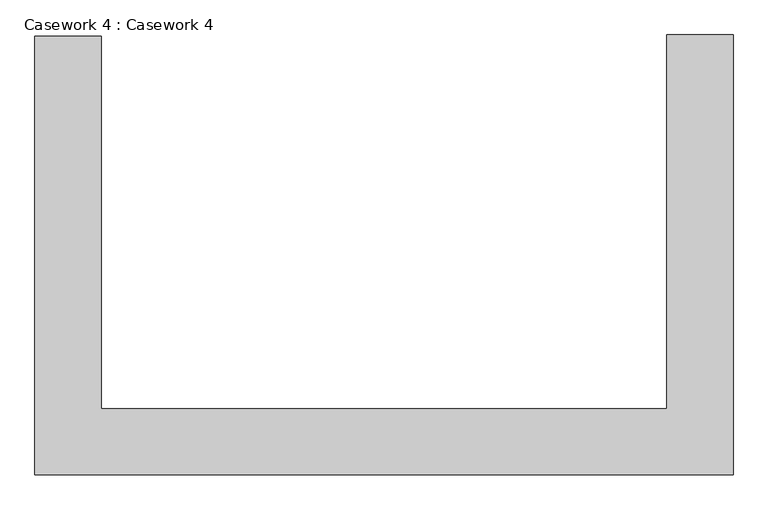
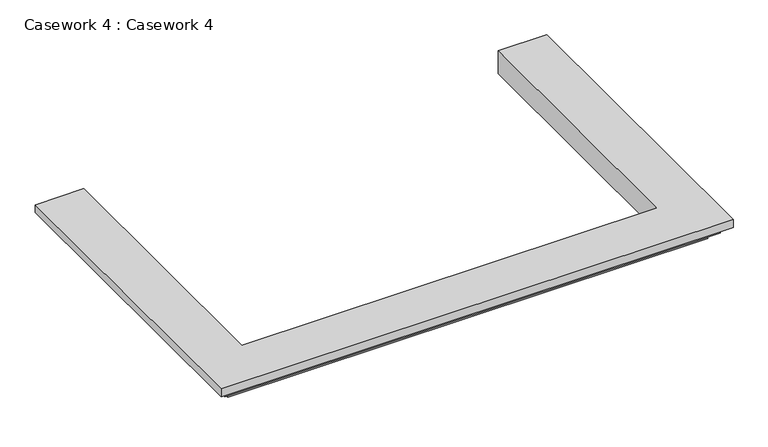
"""IFC4 building model written with IfcOpenShell, lengths in millimetres: furniture geometry, Casework 4 : Casework 4."""

from ifc_helpers import new_model, si_unit, origin, place, context, project, spatial, faceted_brep, source, transform, mapped, element, save


def casework_4_casework_4_96edb60c(model_context):
    return source(origin(), model_context, "Body", "Brep", [
        faceted_brep([(-1879.2953966, -9509.1929163, 4350.0), (-2279.2953966, -9509.1929163, 4350.0), (-2279.2953966, -9509.1929163, 4450.0), (-2379.2953966, -9509.1929163, 4450.0), (-2379.2953966, -9509.1929163, 4550.0), (-2479.2953966, -9509.1929163, 4550.0), (-2479.2953966, -9509.1929163, 4650.0), (-1879.2953966, -9509.1929163, 4650.0), (-1879.2953966, -12886.6929163, 4350.0), (3255.7046034, -12886.6929163, 4350.0), (3255.7046034, -9496.6929163, 4350.0), (3655.7046034, -9496.6929163, 4350.0), (3655.7046034, -13286.6929163, 4350.0), (-2279.2953966, -13286.6929163, 4350.0), (-2279.2953966, -13286.6929163, 4450.0), (3655.7046034, -13286.6929163, 4450.0), (3655.7046034, -9496.6929163, 4450.0), (3755.7046034, -9496.6929163, 4450.0), (3755.7046034, -13386.6929163, 4450.0), (-2379.2953966, -13386.6929163, 4450.0), (-2379.2953966, -13386.6929163, 4550.0), (3755.7046034, -13386.6929163, 4550.0), (3755.7046034, -9496.6929163, 4550.0), (3855.7046034, -9496.6929163, 4550.0), (3855.7046034, -13486.6929163, 4550.0), (-2479.2953966, -13486.6929163, 4550.0), (-2479.2953966, -13486.6929163, 4650.0), (3855.7046034, -13486.6929163, 4650.0), (3855.7046034, -9496.6929163, 4650.0), (3255.7046034, -9496.6929163, 4650.0), (3255.7046034, -12886.6929163, 4650.0), (-1879.2953966, -12886.6929163, 4650.0)], [[[0, 1, 2, 3, 4, 5, 6, 7]], [[1, 0, 8, 9, 10, 11, 12, 13]], [[2, 1, 13, 14]], [[3, 2, 14, 15, 16, 17, 18, 19]], [[4, 3, 19, 20]], [[5, 4, 20, 21, 22, 23, 24, 25]], [[6, 5, 25, 26]], [[7, 6, 26, 27, 28, 29, 30, 31]], [[8, 0, 7, 31]], [[14, 13, 12, 15]], [[20, 19, 18, 21]], [[26, 25, 24, 27]], [[8, 31, 30, 9]], [[16, 15, 12, 11]], [[22, 21, 18, 17]], [[28, 27, 24, 23]], [[10, 9, 30, 29]], [[10, 29, 28, 23, 22, 17, 16, 11]]]),
    ])


if __name__ == "__main__":
    model = new_model("IFC4")
    model_context = context("Model", 3, world=origin())
    ifc_project = project(units=[si_unit("LENGTHUNIT", "METRE", prefix="MILLI")], contexts=[model_context])
    site = spatial("IfcSite", under=ifc_project)
    building = spatial("IfcBuilding", under=site)
    placement = place(None, origin())
    casework_4_casework_4_shape = casework_4_casework_4_96edb60c(model_context)
    element("IfcFurniture", 1, ObjectType="Casework 4 : Casework 4", at=placement, inside=building, context=model_context, shape_type="MappedRepresentation", body=[
        mapped(casework_4_casework_4_shape, transform((0.0, 0.0, 0.0), x_axis=(1.0, 0.0, 0.0), y_axis=(0.0, 1.0, 0.0), z_axis=(0.0, 0.0, 1.0))),
    ])
    save(model, "model.ifc")
